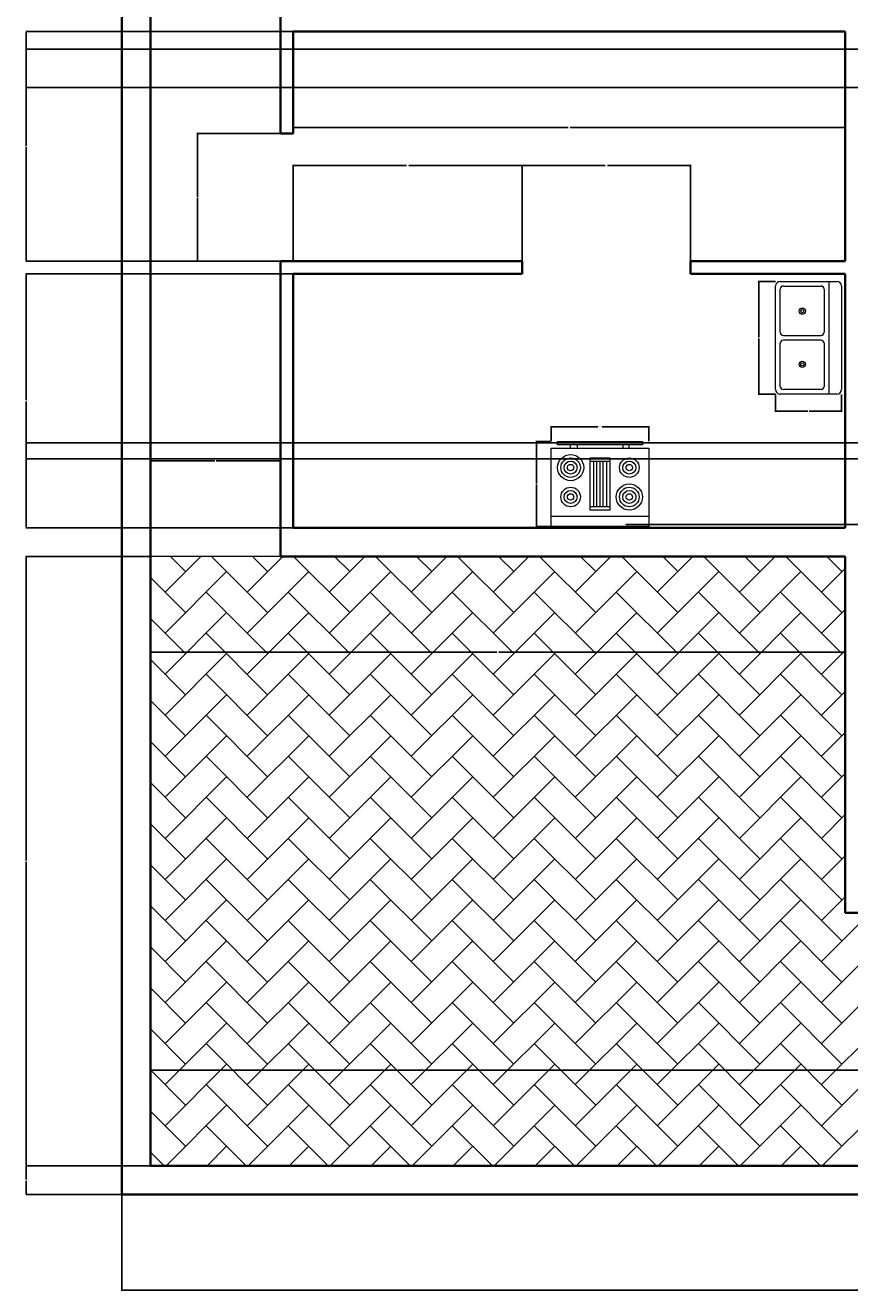
# Model space of a CAD drawing. Units: feet. Extents: x 2335 to 2876, y 491 to 1152.
# Tile 1 of 4: x 2335 to 2595, y 491 to 890. Entities that reach past the tile are written whole.
import ezdxf

# ---------------------------------------------------------------- set-up
doc = ezdxf.new("R2010")
doc.units = ezdxf.units.FT
for name, color, linetype, lineweight in [('A-ANNO-DIMS', 2, 'Continuous', 18), ('A-EQPM', 9, 'Continuous', 18), ('A-FLOR-FIXT', 9, 'Continuous', 18), ('A-WALL', 7, 'Continuous', 35), ('C-PROP', 3, 'Continuous', 35), ('C-PVMT', 8, 'Continuous', 18), ('C-PVMT-PATT', 252, 'Continuous', 13)]:
    doc.layers.add(name, color=color, linetype=linetype, lineweight=lineweight)
doc.styles.get("Standard").update_dxf_attribs({"font": 'arial.ttf'})
doc.dimstyles.get("Standard").update_dxf_attribs({"dimtxt": 0.18, "dimasz": 0.18, "dimexe": 0.18, "dimexo": 0.0625, "dimgap": 0.09, "dimtad": 0, "dimtih": 1, "dimtoh": 1, "dimdec": 4, "dimzin": 0, "dimdsep": 46, "dimlunit": 4, "dimtxsty": 'Standard', "dimcen": 0.09, "dimadec": 0, "dimazin": 0, "dimtfac": 1, "dimtdec": 4, "dimtofl": 0, "dimtmove": 0, "dimatfit": 3, "dimfxl": 1, "dimtolj": 1, "dimtzin": 0, "dimarcsym": 0})

# ---------------------------------------------------------------- blocks, each defined once
blk = doc.blocks.new('Range-Oven - 30 in top')
for p, q in [((0, -3), (30, -3)), ((12, -6), (18, -6)), ((13, -20), (13, -6)), ((14, -6), (14, -20)), ((15, -20), (15, -6)), ((16, -6), (16, -20)), ((17, -20), (17, -6)), ((18, -20), (12, -20)), ((6, -24), (6, -25)), ((8, -25), (8, -24)), ((22, -25), (22, -24)), ((24, -24), (24, -25))]:
    blk.add_line(p, q)
for points in [[(0, -24), (0, 0), (30, 0), (30, -24)], [(12, -21), (12, -5), (18, -5), (18, -21)], [(2, -26), (2, -25), (28, -25), (28, -26)]]:
    blk.add_lwpolyline(points, close=True)
for centre, radius in [((6, -9), 4), ((6, -9), 3), ((6, -9), 2), ((24, -9), 3), ((24, -9), 2), ((6, -9), 1), ((24, -9), 1), ((6, -18), 3), ((24, -18), 4), ((24, -18), 3), ((6, -18), 2), ((6, -18), 1), ((24, -18), 2), ((24, -18), 1)]:
    blk.add_circle(centre, radius)
blk = doc.blocks.new('Sink-double - 36 in top')
for p, q in [((-18, -4), (18, -4)), ((-0.75, -18.5), (-0.75, -6.5)), ((0.75, -6.5), (0.75, -18.5))]:
    blk.add_line(p, q)
for points in [[(-16.5, 0), (16.5, 0)], [(-18, -19.5), (-18, -1.5)], [(18, -1.5), (18, -19.5)], [(-16.5, -18.5), (-16.5, -6.5)], [(-15.5, -5.5), (-1.75, -5.5)], [(1.75, -5.5), (15.5, -5.5)], [(16.5, -6.5), (16.5, -18.5)], [(-1.75, -19.5), (-15.5, -19.5)], [(15.5, -19.5), (1.75, -19.5)], [(16.5, -21), (-16.5, -21)]]:
    blk.add_lwpolyline(points)
for centre, radius in [((-8.5, -12.5), 1), ((-8.5, -12.5), 0.5), ((8.5, -12.5), 1), ((8.5, -12.5), 0.5)]:
    blk.add_circle(centre, radius)
for centre, radius, start, end in [((-16.5, -1.5), 1.5, 90, 180), ((16.5, -1.5), 1.5, 0, 90), ((-15.5, -6.5), 1, 90, 180), ((-1.75, -6.5), 1, 0, 90), ((1.75, -6.5), 1, 90, 180), ((15.5, -6.5), 1, 0, 90), ((-16.5, -19.5), 1.5, 180, 270), ((-15.5, -18.5), 1, 180, 270), ((-1.75, -18.5), 1, 270, 0), ((1.75, -18.5), 1, 180, 270), ((15.5, -18.5), 1, 270, 0), ((16.5, -19.5), 1.5, 270, 0)]:
    blk.add_arc(centre, radius, start, end)
blk = doc.blocks.new('*D16')
at = {"layer": 'A-ANNO-DIMS', "color": 0, "lineweight": -2, "transparency": 16777216}
for p, q in [((2501.1, 758.74), (2501.1, 763.48)), ((2501.28, 763.3), (2515.84, 763.3)), ((2531.75, 763.3), (2517.2, 763.3)), ((2531.93, 758.74), (2531.93, 763.48))]:
    blk.add_line(p, q, dxfattribs=at)
at = {"layer": 'A-ANNO-DIMS', "color": 0, "transparency": 16777216}
for points in [[(2501.28, 763.33), (2501.28, 763.27), (2501.1, 763.3)], [(2531.75, 763.33), (2531.75, 763.27), (2531.93, 763.3)]]:
    blk.add_solid(points, dxfattribs=at)
at = {"layer": 'Defpoints', "color": 0, "transparency": 16777216}
for p in [(2501.1, 763.3), (2501.1, 758.68), (2531.93, 758.68)]:
    blk.add_point(p, dxfattribs=at)
at = {"layer": 'A-ANNO-DIMS', "color": 0, "transparency": 16777216, "insert": (2516.52, 763.3), "char_height": 0.18, "attachment_point": 5}
blk.add_mtext('\\A1;RANGE 31', dxfattribs=at)
blk = doc.blocks.new('*D17')
at = {"layer": 'A-ANNO-DIMS', "color": 0, "lineweight": -2, "transparency": 16777216}
for p, q in [((2501.04, 758.68), (2496.29, 758.68)), ((2496.47, 758.5), (2496.47, 745.5)), ((2496.47, 732.13), (2496.47, 745.14)), ((2501.04, 731.95), (2496.29, 731.95))]:
    blk.add_line(p, q, dxfattribs=at)
at = {"layer": 'A-ANNO-DIMS', "color": 0, "transparency": 16777216}
for points in [[(2496.44, 758.5), (2496.5, 758.5), (2496.47, 758.68)], [(2496.44, 732.13), (2496.5, 732.13), (2496.47, 731.95)]]:
    blk.add_solid(points, dxfattribs=at)
at = {"layer": 'Defpoints', "color": 0, "transparency": 16777216}
for p in [(2501.1, 758.68), (2496.47, 731.95), (2501.1, 731.95)]:
    blk.add_point(p, dxfattribs=at)
at = {"layer": 'A-ANNO-DIMS', "color": 0, "transparency": 16777216, "insert": (2496.47, 745.32), "char_height": 0.18, "attachment_point": 5}
blk.add_mtext('\\A1;27', dxfattribs=at)
blk = doc.blocks.new('*D18')
at = {"layer": 'A-ANNO-DIMS', "color": 0, "lineweight": -2, "transparency": 16777216}
for p, q in [((2571.83, 809.13), (2566.38, 809.13)), ((2566.56, 808.95), (2566.56, 791.54)), ((2566.56, 773.77), (2566.56, 791.18)), ((2571.83, 773.59), (2566.38, 773.59))]:
    blk.add_line(p, q, dxfattribs=at)
at = {"layer": 'A-ANNO-DIMS', "color": 0, "transparency": 16777216}
for points in [[(2566.53, 808.95), (2566.59, 808.95), (2566.56, 809.13)], [(2566.53, 773.77), (2566.59, 773.77), (2566.56, 773.59)]]:
    blk.add_solid(points, dxfattribs=at)
at = {"layer": 'Defpoints', "color": 0, "transparency": 16777216}
for p in [(2571.89, 809.13), (2566.56, 773.59), (2571.89, 773.59)]:
    blk.add_point(p, dxfattribs=at)
at = {"layer": 'A-ANNO-DIMS', "color": 0, "transparency": 16777216, "insert": (2566.56, 791.36), "char_height": 0.18, "attachment_point": 5}
blk.add_mtext('\\A1;SINK 36', dxfattribs=at)
blk = doc.blocks.new('*D19')
at = {"layer": 'A-ANNO-DIMS', "color": 0, "lineweight": -2, "transparency": 16777216}
for p, q in [((2571.89, 773.52), (2571.89, 768.07)), ((2592.63, 773.52), (2592.63, 768.07)), ((2572.07, 768.25), (2582.05, 768.25)), ((2592.45, 768.25), (2582.46, 768.25))]:
    blk.add_line(p, q, dxfattribs=at)
at = {"layer": 'A-ANNO-DIMS', "color": 0, "transparency": 16777216}
for points in [[(2572.07, 768.28), (2572.07, 768.22), (2571.89, 768.25)], [(2592.45, 768.28), (2592.45, 768.22), (2592.63, 768.25)]]:
    blk.add_solid(points, dxfattribs=at)
at = {"layer": 'Defpoints', "color": 0, "transparency": 16777216}
for p in [(2571.89, 773.59), (2592.63, 773.59), (2592.63, 768.25)]:
    blk.add_point(p, dxfattribs=at)
at = {"layer": 'A-ANNO-DIMS', "color": 0, "transparency": 16777216, "insert": (2582.26, 768.25), "char_height": 0.18, "attachment_point": 5}
blk.add_mtext('\\A1;21', dxfattribs=at)
blk = doc.blocks.new('*D24')
at = {"layer": 'A-ANNO-DIMS', "color": 0, "lineweight": -2, "transparency": 16777216}
for p, q in [((2365.8, 521.42), (2365.8, 491.16)), ((2845.8, 521.42), (2845.8, 491.16)), ((2365.98, 491.34), (2605.5, 491.34)), ((2845.62, 491.34), (2606.09, 491.34))]:
    blk.add_line(p, q, dxfattribs=at)
at = {"layer": 'A-ANNO-DIMS', "color": 0, "transparency": 16777216}
for points in [[(2365.98, 491.37), (2365.98, 491.31), (2365.8, 491.34)], [(2845.62, 491.37), (2845.62, 491.31), (2845.8, 491.34)]]:
    blk.add_solid(points, dxfattribs=at)
at = {"layer": 'Defpoints', "color": 0, "transparency": 16777216}
for p in [(2365.8, 521.49), (2845.8, 521.49), (2845.8, 491.34)]:
    blk.add_point(p, dxfattribs=at)
at = {"layer": 'A-ANNO-DIMS', "color": 0, "transparency": 16777216, "insert": (2605.8, 491.34), "char_height": 0.18, "attachment_point": 5}
blk.add_mtext('\\A1;480', dxfattribs=at)
blk = doc.blocks.new('*D26')
at = {"layer": 'A-ANNO-DIMS', "color": 0, "lineweight": -2, "transparency": 16777216}
for p, q in [((2374.8, 530.55), (2374.8, 560.82)), ((2374.98, 560.64), (2605.51, 560.64)), ((2836.62, 560.64), (2606.09, 560.64)), ((2836.8, 530.55), (2836.8, 560.82))]:
    blk.add_line(p, q, dxfattribs=at)
at = {"layer": 'A-ANNO-DIMS', "color": 0, "transparency": 16777216}
for points in [[(2374.98, 560.67), (2374.98, 560.61), (2374.8, 560.64)], [(2836.62, 560.67), (2836.62, 560.61), (2836.8, 560.64)]]:
    blk.add_solid(points, dxfattribs=at)
at = {"layer": 'Defpoints', "color": 0, "transparency": 16777216}
for p in [(2836.8, 560.64), (2374.8, 530.49), (2836.8, 530.49)]:
    blk.add_point(p, dxfattribs=at)
at = {"layer": 'A-ANNO-DIMS', "color": 0, "transparency": 16777216, "insert": (2605.8, 560.64), "char_height": 0.18, "attachment_point": 5}
blk.add_mtext('\\A1;462', dxfattribs=at)
blk = doc.blocks.new('*D27')
at = {"layer": 'A-ANNO-DIMS', "color": 0, "lineweight": -2, "transparency": 16777216}
for p, q in [((2374.8, 722.42), (2374.8, 692.16)), ((2593.8, 722.42), (2593.8, 692.16)), ((2374.98, 692.34), (2484.01, 692.34)), ((2593.62, 692.34), (2484.59, 692.34))]:
    blk.add_line(p, q, dxfattribs=at)
at = {"layer": 'A-ANNO-DIMS', "color": 0, "transparency": 16777216}
for points in [[(2374.98, 692.37), (2374.98, 692.31), (2374.8, 692.34)], [(2593.62, 692.37), (2593.62, 692.31), (2593.8, 692.34)]]:
    blk.add_solid(points, dxfattribs=at)
at = {"layer": 'Defpoints', "color": 0, "transparency": 16777216}
for p in [(2374.8, 722.49), (2593.8, 722.49), (2374.8, 692.34)]:
    blk.add_point(p, dxfattribs=at)
at = {"layer": 'A-ANNO-DIMS', "color": 0, "transparency": 16777216, "insert": (2484.3, 692.34), "char_height": 0.18, "attachment_point": 5}
blk.add_mtext('\\A1;219', dxfattribs=at)
blk = doc.blocks.new('*D28')
at = {"layer": 'A-ANNO-DIMS', "color": 0, "lineweight": -2, "transparency": 16777216}
for p, q in [((2374.73, 722.49), (2335.47, 722.49)), ((2335.65, 722.31), (2335.65, 626.67)), ((2335.65, 530.67), (2335.65, 626.31)), ((2374.73, 530.49), (2335.47, 530.49))]:
    blk.add_line(p, q, dxfattribs=at)
at = {"layer": 'A-ANNO-DIMS', "color": 0, "transparency": 16777216}
for points in [[(2335.62, 722.31), (2335.68, 722.31), (2335.65, 722.49)], [(2335.62, 530.67), (2335.68, 530.67), (2335.65, 530.49)]]:
    blk.add_solid(points, dxfattribs=at)
at = {"layer": 'Defpoints', "color": 0, "transparency": 16777216}
for p in [(2335.65, 722.49), (2374.8, 722.49), (2374.8, 530.49)]:
    blk.add_point(p, dxfattribs=at)
at = {"layer": 'A-ANNO-DIMS', "color": 0, "transparency": 16777216, "insert": (2335.65, 626.49), "char_height": 0.18, "attachment_point": 5}
blk.add_mtext('\\A1;192', dxfattribs=at)
blk = doc.blocks.new('*D29')
at = {"layer": 'A-ANNO-DIMS', "color": 0, "lineweight": -2, "transparency": 16777216}
for p, q in [((2374.73, 530.49), (2335.47, 530.49)), ((2335.65, 530.31), (2335.65, 526.17)), ((2335.65, 521.67), (2335.65, 525.81)), ((2365.73, 521.49), (2335.47, 521.49))]:
    blk.add_line(p, q, dxfattribs=at)
at = {"layer": 'A-ANNO-DIMS', "color": 0, "transparency": 16777216}
for points in [[(2335.62, 530.31), (2335.68, 530.31), (2335.65, 530.49)], [(2335.62, 521.67), (2335.68, 521.67), (2335.65, 521.49)]]:
    blk.add_solid(points, dxfattribs=at)
at = {"layer": 'Defpoints', "color": 0, "transparency": 16777216}
for p in [(2335.65, 530.49), (2374.8, 530.49), (2365.8, 521.49)]:
    blk.add_point(p, dxfattribs=at)
at = {"layer": 'A-ANNO-DIMS', "color": 0, "transparency": 16777216, "insert": (2335.65, 525.99), "char_height": 0.18, "attachment_point": 5}
blk.add_mtext('\\A1;9', dxfattribs=at)
blk = doc.blocks.new('*D39')
at = {"layer": 'A-ANNO-DIMS', "color": 0, "lineweight": -2, "transparency": 16777216}
for p, q in [((2760.82, 882.23), (2335.47, 882.23)), ((2335.65, 882.05), (2335.65, 876.41)), ((2335.65, 870.41), (2335.65, 876.05)), ((2760.82, 870.23), (2335.47, 870.23))]:
    blk.add_line(p, q, dxfattribs=at)
at = {"layer": 'A-ANNO-DIMS', "color": 0, "transparency": 16777216}
for points in [[(2335.62, 882.05), (2335.68, 882.05), (2335.65, 882.23)], [(2335.62, 870.41), (2335.68, 870.41), (2335.65, 870.23)]]:
    blk.add_solid(points, dxfattribs=at)
at = {"layer": 'Defpoints', "color": 0, "transparency": 16777216}
for p in [(2335.65, 882.23), (2760.88, 882.23), (2760.88, 870.23)]:
    blk.add_point(p, dxfattribs=at)
at = {"layer": 'A-ANNO-DIMS', "color": 0, "transparency": 16777216, "insert": (2335.65, 876.23), "char_height": 0.18, "attachment_point": 5}
blk.add_mtext('\\A1;12', dxfattribs=at)
blk = doc.blocks.new('*D43')
at = {"layer": 'A-ANNO-DIMS', "color": 0, "lineweight": -2, "transparency": 16777216}
for p, q in [((2760.82, 758.23), (2335.47, 758.23)), ((2335.65, 758.05), (2335.65, 755.91)), ((2335.65, 753.41), (2335.65, 755.54)), ((2760.82, 753.23), (2335.47, 753.23))]:
    blk.add_line(p, q, dxfattribs=at)
at = {"layer": 'A-ANNO-DIMS', "color": 0, "transparency": 16777216}
for points in [[(2335.62, 758.05), (2335.68, 758.05), (2335.65, 758.23)], [(2335.62, 753.41), (2335.68, 753.41), (2335.65, 753.23)]]:
    blk.add_solid(points, dxfattribs=at)
at = {"layer": 'Defpoints', "color": 0, "transparency": 16777216}
for p in [(2335.65, 758.23), (2760.88, 758.23), (2760.88, 753.23)]:
    blk.add_point(p, dxfattribs=at)
at = {"layer": 'A-ANNO-DIMS', "color": 0, "transparency": 16777216, "insert": (2335.65, 755.73), "char_height": 0.18, "attachment_point": 5}
blk.add_mtext('\\A1;5', dxfattribs=at)
blk = doc.blocks.new('*D44')
at = {"layer": 'A-ANNO-DIMS', "color": 0, "lineweight": -2, "transparency": 16777216}
for p, q in [((2374.8, 722.55), (2374.8, 752.82)), ((2374.98, 752.64), (2395.09, 752.64)), ((2415.62, 752.64), (2395.5, 752.64)), ((2415.8, 722.55), (2415.8, 752.82))]:
    blk.add_line(p, q, dxfattribs=at)
at = {"layer": 'A-ANNO-DIMS', "color": 0, "transparency": 16777216}
for points in [[(2374.98, 752.67), (2374.98, 752.61), (2374.8, 752.64)], [(2415.62, 752.67), (2415.62, 752.61), (2415.8, 752.64)]]:
    blk.add_solid(points, dxfattribs=at)
at = {"layer": 'Defpoints', "color": 0, "transparency": 16777216}
for p in [(2415.8, 752.64), (2374.8, 722.49), (2415.8, 722.49)]:
    blk.add_point(p, dxfattribs=at)
at = {"layer": 'A-ANNO-DIMS', "color": 0, "transparency": 16777216, "insert": (2395.3, 752.64), "char_height": 0.18, "attachment_point": 5}
blk.add_mtext('\\A1;41', dxfattribs=at)
blk = doc.blocks.new('*D45')
at = {"layer": 'A-ANNO-DIMS', "color": 0, "lineweight": -2, "transparency": 16777216}
for p, q in [((2419.73, 811.49), (2335.47, 811.49)), ((2335.65, 811.31), (2335.65, 771.67)), ((2335.65, 731.67), (2335.65, 771.31)), ((2419.73, 731.49), (2335.47, 731.49))]:
    blk.add_line(p, q, dxfattribs=at)
at = {"layer": 'A-ANNO-DIMS', "color": 0, "transparency": 16777216}
for points in [[(2335.62, 811.31), (2335.68, 811.31), (2335.65, 811.49)], [(2335.62, 731.67), (2335.68, 731.67), (2335.65, 731.49)]]:
    blk.add_solid(points, dxfattribs=at)
at = {"layer": 'Defpoints', "color": 0, "transparency": 16777216}
for p in [(2335.65, 811.49), (2419.8, 811.49), (2419.8, 731.49)]:
    blk.add_point(p, dxfattribs=at)
at = {"layer": 'A-ANNO-DIMS', "color": 0, "transparency": 16777216, "insert": (2335.65, 771.49), "char_height": 0.18, "attachment_point": 5}
blk.add_mtext('\\A1;80', dxfattribs=at)
blk = doc.blocks.new('*D46')
at = {"layer": 'A-ANNO-DIMS', "color": 0, "lineweight": -2, "transparency": 16777216}
for p, q in [((2419.8, 815.55), (2419.8, 845.82)), ((2419.98, 845.64), (2455.53, 845.64)), ((2491.83, 845.64), (2456.28, 845.64)), ((2492.01, 815.55), (2492.01, 845.82))]:
    blk.add_line(p, q, dxfattribs=at)
at = {"layer": 'A-ANNO-DIMS', "color": 0, "transparency": 16777216}
for points in [[(2419.98, 845.67), (2419.98, 845.61), (2419.8, 845.64)], [(2491.83, 845.67), (2491.83, 845.61), (2492.01, 845.64)]]:
    blk.add_solid(points, dxfattribs=at)
at = {"layer": 'Defpoints', "color": 0, "transparency": 16777216}
for p in [(2492.01, 845.64), (2419.8, 815.49), (2492.01, 815.49)]:
    blk.add_point(p, dxfattribs=at)
at = {"layer": 'A-ANNO-DIMS', "color": 0, "transparency": 16777216, "insert": (2455.9, 845.64), "char_height": 0.18, "attachment_point": 5}
blk.add_mtext('\\A1;72.21', dxfattribs=at)
blk = doc.blocks.new('*D47')
at = {"layer": 'A-ANNO-DIMS', "color": 0, "lineweight": -2, "transparency": 16777216}
for p, q in [((2492.01, 815.55), (2492.01, 845.82)), ((2492.19, 845.64), (2518.14, 845.64)), ((2544.88, 845.64), (2518.92, 845.64)), ((2545.06, 815.55), (2545.06, 845.82))]:
    blk.add_line(p, q, dxfattribs=at)
at = {"layer": 'A-ANNO-DIMS', "color": 0, "transparency": 16777216}
for points in [[(2492.19, 845.67), (2492.19, 845.61), (2492.01, 845.64)], [(2544.88, 845.67), (2544.88, 845.61), (2545.06, 845.64)]]:
    blk.add_solid(points, dxfattribs=at)
at = {"layer": 'Defpoints', "color": 0, "transparency": 16777216}
for p in [(2545.06, 845.64), (2492.01, 815.49), (2545.06, 815.49)]:
    blk.add_point(p, dxfattribs=at)
at = {"layer": 'A-ANNO-DIMS', "color": 0, "transparency": 16777216, "insert": (2518.53, 845.64), "char_height": 0.18, "attachment_point": 5}
blk.add_mtext('\\A1;53.05', dxfattribs=at)
blk = doc.blocks.new('*D48')
at = {"layer": 'A-ANNO-DIMS', "color": 0, "lineweight": -2, "transparency": 16777216}
for p, q in [((2419.73, 887.8), (2335.47, 887.8)), ((2335.65, 887.62), (2335.65, 851.82)), ((2335.65, 815.67), (2335.65, 851.46)), ((2419.73, 815.49), (2335.47, 815.49))]:
    blk.add_line(p, q, dxfattribs=at)
at = {"layer": 'A-ANNO-DIMS', "color": 0, "transparency": 16777216}
for points in [[(2335.62, 887.62), (2335.68, 887.62), (2335.65, 887.8)], [(2335.62, 815.67), (2335.68, 815.67), (2335.65, 815.49)]]:
    blk.add_solid(points, dxfattribs=at)
at = {"layer": 'Defpoints', "color": 0, "transparency": 16777216}
for p in [(2335.65, 887.8), (2419.8, 887.8), (2419.8, 815.49)]:
    blk.add_point(p, dxfattribs=at)
at = {"layer": 'A-ANNO-DIMS', "color": 0, "transparency": 16777216, "insert": (2335.65, 851.64), "char_height": 0.18, "attachment_point": 5}
blk.add_mtext('\\A1;72.31', dxfattribs=at)
blk = doc.blocks.new('*D49')
at = {"layer": 'A-ANNO-DIMS', "color": 0, "lineweight": -2, "transparency": 16777216}
for p, q in [((2419.73, 855.76), (2389.47, 855.76)), ((2389.65, 855.58), (2389.65, 835.8)), ((2389.65, 815.67), (2389.65, 835.44)), ((2419.73, 815.49), (2389.47, 815.49))]:
    blk.add_line(p, q, dxfattribs=at)
at = {"layer": 'A-ANNO-DIMS', "color": 0, "transparency": 16777216}
for points in [[(2389.68, 855.58), (2389.62, 855.58), (2389.65, 855.76)], [(2389.68, 815.67), (2389.62, 815.67), (2389.65, 815.49)]]:
    blk.add_solid(points, dxfattribs=at)
at = {"layer": 'Defpoints', "color": 0, "transparency": 16777216}
for p in [(2389.65, 855.76), (2419.8, 855.76), (2419.8, 815.49)]:
    blk.add_point(p, dxfattribs=at)
at = {"layer": 'A-ANNO-DIMS', "color": 0, "transparency": 16777216, "insert": (2389.65, 835.62), "char_height": 0.18, "attachment_point": 5}
blk.add_mtext('\\A1;40.27', dxfattribs=at)
blk = doc.blocks.new('*D54')
at = {"layer": 'A-ANNO-DIMS', "color": 0, "lineweight": -2, "transparency": 16777216}
for p, q in [((2419.8, 887.74), (2419.8, 857.47)), ((2593.8, 887.74), (2593.8, 857.47)), ((2419.98, 857.65), (2506.52, 857.65)), ((2593.62, 857.65), (2507.08, 857.65))]:
    blk.add_line(p, q, dxfattribs=at)
at = {"layer": 'A-ANNO-DIMS', "color": 0, "transparency": 16777216}
for points in [[(2419.98, 857.68), (2419.98, 857.62), (2419.8, 857.65)], [(2593.62, 857.68), (2593.62, 857.62), (2593.8, 857.65)]]:
    blk.add_solid(points, dxfattribs=at)
at = {"layer": 'Defpoints', "color": 0, "transparency": 16777216}
for p in [(2419.8, 887.8), (2593.8, 887.8), (2419.8, 857.65)]:
    blk.add_point(p, dxfattribs=at)
at = {"layer": 'A-ANNO-DIMS', "color": 0, "transparency": 16777216, "insert": (2506.8, 857.65), "char_height": 0.18, "attachment_point": 5}
blk.add_mtext('\\A1;174', dxfattribs=at)
blk = doc.blocks.new('*D70')
at = {"layer": 'A-ANNO-DIMS', "color": 0, "lineweight": -2, "transparency": 16777216}
for p, q in [((2526.66, 732.49), (2605.99, 732.49)), ((2738.6, 732.49), (2738.78, 732.49)), ((2738.69, 732.4), (2738.69, 732.58))]:
    blk.add_line(p, q, dxfattribs=at)
at = {"layer": 'A-ANNO-DIMS', "color": 0, "transparency": 16777216}
blk.add_solid([(2605.99, 732.52), (2605.99, 732.46), (2606.17, 732.49)], dxfattribs=at)
at = {"layer": 'Defpoints', "color": 0, "transparency": 16777216}
for p in [(2606.17, 732.49), (2738.69, 732.49)]:
    blk.add_point(p, dxfattribs=at)
at = {"layer": 'A-ANNO-DIMS', "color": 0, "transparency": 16777216, "insert": (2526.11, 732.49), "char_height": 0.18, "attachment_point": 5}
blk.add_mtext('\\A1;R132.52', dxfattribs=at)
blk = doc.blocks.new('*D71')
at = {"layer": 'A-ANNO-DIMS', "color": 0, "lineweight": -2, "transparency": 16777216}
for p, q in [((2524.65, 732.49), (2599.43, 732.49)), ((2724.44, 732.49), (2724.62, 732.49)), ((2724.53, 732.4), (2724.53, 732.58))]:
    blk.add_line(p, q, dxfattribs=at)
at = {"layer": 'A-ANNO-DIMS', "color": 0, "transparency": 16777216}
blk.add_solid([(2599.43, 732.52), (2599.43, 732.46), (2599.61, 732.49)], dxfattribs=at)
at = {"layer": 'Defpoints', "color": 0, "transparency": 16777216}
for p in [(2599.61, 732.49), (2724.53, 732.49)]:
    blk.add_point(p, dxfattribs=at)
at = {"layer": 'A-ANNO-DIMS', "color": 0, "transparency": 16777216, "insert": (2524.1, 732.49), "char_height": 0.18, "attachment_point": 5}
blk.add_mtext('\\A1;R124.93', dxfattribs=at)

msp = doc.modelspace()

# ---------------------------------------------------------------- hatches: boundary and pattern name
at = {"layer": 'C-PVMT-PATT'}
h = msp.add_hatch(dxfattribs=at)
h.set_pattern_fill('AR-HBONE', color=256, scale=0.09)
h.paths.add_polyline_path([(2593.7974, 722.4872), (2419.7974, 722.4872), (2415.7974, 722.4872), (2374.7967, 722.4872), (2374.7967, 530.4872), (2593.7974, 530.4872), (2597.7974, 530.4872), (2836.7967, 530.4872), (2836.7967, 610.2261), (2729.1837, 610.2261), (2652.5752, 610.2261), (2597.7974, 610.2261), (2593.7974, 610.2261)])

# ---------------------------------------------------------------- linework, layer by layer
at = {"layer": 'A-WALL'}
for p, q in [((2415.7974, 855.7568), (2415.7974, 1081.7975)), ((2419.7969, 855.7568), (2419.7969, 887.7975)), ((2419.7974, 887.7975), (2593.7974, 887.7975)), ((2593.7974, 887.7975), (2593.7974, 815.4872)), ((2415.7974, 855.7568), (2419.7969, 855.7568)), ((2415.7974, 722.4872), (2415.7974, 815.4872)), ((2419.7967, 815.4872), (2415.7974, 815.4872)), ((2419.7974, 815.4872), (2492.0051, 815.4872)), ((2464.7974, 815.4872), (2492.0051, 815.4872)), ((2492.0051, 811.4872), (2492.0051, 815.4872)), ((2545.0559, 815.4872), (2545.0559, 811.4872)), ((2545.0559, 815.4872), (2593.7974, 815.4872)), ((2545.0559, 815.4872), (2593.7974, 815.4872)), ((2419.7974, 811.4872), (2492.0051, 811.4872)), ((2419.7974, 811.4872), (2419.7974, 731.4872)), ((2545.0559, 811.4872), (2593.7974, 811.4872)), ((2593.7974, 811.4872), (2593.7974, 731.4872)), ((2593.7974, 811.4872), (2593.7974, 784.7975)), ((2419.7974, 731.4872), (2593.7974, 731.4872)), ((2419.7974, 722.4872), (2415.7974, 722.4872)), ((2593.7974, 722.4872), (2419.7974, 722.4872)), ((2593.7974, 722.4872), (2593.7974, 610.2261)), ((2597.7974, 610.2261), (2593.7974, 610.2261))]:
    msp.add_line(p, q, dxfattribs=at)
at = {"layer": 'C-PROP'}
msp.add_line((2593.7974, 530.4872), (2597.7974, 530.4872), dxfattribs=at)
msp.add_lwpolyline([(2845.7967, 521.4872), (2845.7967, 1121.4872), (2365.7967, 1121.4872), (2365.7967, 521.4872)], close=True, dxfattribs=at)
msp.add_lwpolyline([(2697.7974, 1112.4872), (2374.7967, 1112.4872), (2374.7967, 530.4872), (2593.7974, 530.4872)], dxfattribs=at)
at = {"layer": 'C-PVMT'}
msp.add_line((2415.7974, 722.4872), (2374.7967, 722.4872), dxfattribs=at)

# ---------------------------------------------------------------- block references
at = {"layer": 'A-EQPM', "xscale": 1.027898850187762, "yscale": 1.027898850187762, "zscale": 1.027898850187762, "rotation": 180}
msp.add_blockref('Range-Oven - 30 in top', (2531.935, 731.9529), dxfattribs=at)
at = {"layer": 'A-FLOR-FIXT', "xscale": 0.9874339846236208, "yscale": 0.9874339846236208, "zscale": 0.9874339846236208, "rotation": 270}
msp.add_blockref('Sink-double - 36 in top', (2592.6259, 791.3588), dxfattribs=at)

# ---------------------------------------------------------------- dimensions: what is measured, and where the dimension line sits
at = {"layer": 'A-ANNO-DIMS'}
for base, p1, p2, angle, override, picture, middle in [((2335.6467, 887.7975), (2419.7974, 815.4872), (2419.7974, 887.7975), 90, {"dimdec": 2, "dimlfac": 1, "dimrnd": 0, "dimzin": 0, "dimdsep": 46, "dimlunit": 2}, '*D48', (2335.6467, 851.6423)), ((2419.7974, 857.6475), (2593.7974, 887.7975), (2419.7974, 887.7975), 180, {"dimdec": 0, "dimlfac": 1, "dimrnd": 0, "dimzin": 0, "dimdsep": 46, "dimlunit": 2}, '*D54', (2506.7974, 857.6475)), ((2335.6467, 882.2261), (2760.8783, 870.2261), (2760.8783, 882.2261), 90, {"dimdec": 0, "dimlfac": 1, "dimrnd": 0, "dimzin": 0, "dimdsep": 46, "dimlunit": 2}, '*D39', (2335.6467, 876.2261)), ((2389.6469, 855.7564), (2419.7974, 815.4872), (2419.7969, 855.7568), 90.00067, {"dimdec": 2, "dimlfac": 1, "dimrnd": 0, "dimzin": 0, "dimdsep": 46, "dimlunit": 2}, '*D49', (2389.6472, 835.6216)), ((2335.6467, 811.4872), (2419.7974, 731.4872), (2419.7974, 811.4872), 90, {"dimdec": 0, "dimlfac": 1, "dimrnd": 0, "dimzin": 0, "dimdsep": 46, "dimlunit": 2}, '*D45', (2335.6467, 771.4872)), ((2335.6467, 758.2261), (2760.8783, 753.2261), (2760.8783, 758.2261), 90, {"dimdec": 0, "dimlfac": 1, "dimrnd": 0, "dimzin": 0, "dimdsep": 46, "dimlunit": 2}, '*D43', (2335.6467, 755.7261)), ((2496.4725, 731.9529), (2501.098, 758.6783), (2501.098, 731.9529), 270, {"dimdec": 0, "dimlfac": 1, "dimrnd": 0, "dimzin": 0, "dimdsep": 46, "dimlunit": 2}, '*D17', (2496.4725, 745.3156)), ((2335.6467, 722.4872), (2374.7967, 530.4872), (2374.7967, 722.4872), 90, {"dimdec": 0, "dimlfac": 1, "dimrnd": 0, "dimzin": 0, "dimdsep": 46, "dimlunit": 2}, '*D28', (2335.6467, 626.4872)), ((2374.7967, 692.3372), (2593.7974, 722.4872), (2374.7967, 722.4872), 180, {"dimdec": 0, "dimlfac": 1, "dimrnd": 0, "dimzin": 0, "dimdsep": 46, "dimlunit": 2}, '*D27', (2484.297, 692.3372)), ((2836.7967, 560.6372), (2374.7967, 530.4872), (2836.7967, 530.4872), 0, {"dimdec": 0, "dimlfac": 1, "dimrnd": 0, "dimzin": 0, "dimdsep": 46, "dimlunit": 2}, '*D26', (2605.7967, 560.6372)), ((2335.6467, 530.4872), (2365.7967, 521.4872), (2374.7967, 530.4872), 90, {"dimdec": 0, "dimlfac": 1, "dimrnd": 0, "dimzin": 0, "dimdsep": 46, "dimlunit": 2}, '*D29', (2335.6467, 525.9872))]:
    dim = msp.add_linear_dim(base=base, p1=p1, p2=p2, angle=angle, dimstyle='Standard', override=override, dxfattribs=at)
    dim.commit()
    dim.dimension.update_dxf_attribs({"geometry": picture, "text_midpoint": middle})
for base, p1, p2, override, picture, middle in [((2492.0051, 845.6372), (2419.7974, 815.4872), (2492.0051, 815.4872), {"dimdec": 2, "dimlfac": 1, "dimrnd": 0, "dimzin": 0, "dimdsep": 46, "dimlunit": 2}, '*D46', (2455.9013, 845.6372)), ((2545.0559, 845.6372), (2492.0051, 815.4872), (2545.0559, 815.4872), {"dimdec": 2, "dimlfac": 1, "dimrnd": 0, "dimzin": 0, "dimdsep": 46, "dimlunit": 2}, '*D47', (2518.5305, 845.6372)), ((2592.6259, 768.2529), (2571.8897, 773.585), (2592.6259, 773.585), {"dimdec": 0, "dimlfac": 1, "dimrnd": 0, "dimzin": 0, "dimdsep": 46, "dimlunit": 2}, '*D19', (2582.2578, 768.2529)), ((2415.7974, 752.6372), (2374.7967, 722.4872), (2415.7974, 722.4872), {"dimdec": 0, "dimlfac": 1, "dimrnd": 0, "dimzin": 0, "dimdsep": 46, "dimlunit": 2}, '*D44', (2395.297, 752.6372)), ((2845.7967, 491.3372), (2365.7967, 521.4872), (2845.7967, 521.4872), {"dimdec": 0, "dimlfac": 1, "dimrnd": 0, "dimzin": 0, "dimdsep": 46, "dimlunit": 2}, '*D24', (2605.7967, 491.3372))]:
    dim = msp.add_linear_dim(base=base, p1=p1, p2=p2, dimstyle='Standard', override=override, dxfattribs=at)
    dim.commit()
    dim.dimension.update_dxf_attribs({"geometry": picture, "text_midpoint": middle})
for base, p1, p2, angle, text, picture, middle in [((2566.5576, 773.585), (2571.8897, 809.1326), (2571.8897, 773.585), 270, 'SINK <>', '*D18', (2566.5576, 791.3588)), ((2501.098, 763.3038), (2531.935, 758.6783), (2501.098, 758.6783), 180, 'RANGE <>', '*D16', (2516.5165, 763.3038))]:
    dim = msp.add_linear_dim(base=base, p1=p1, p2=p2, angle=angle, text=text, dimstyle='Standard', override={"dimdec": 0, "dimlfac": 1, "dimrnd": 0, "dimzin": 0, "dimdsep": 46, "dimlunit": 2}, dxfattribs=at)
    dim.commit()
    dim.dimension.update_dxf_attribs({"geometry": picture, "text_midpoint": middle})
for center, mpoint, picture, middle in [((2724.5349, 732.4927), (2599.6087, 732.493), '*D71', (2524.6529, 732.4932)), ((2738.6915, 732.4927), (2606.1693, 732.493), '*D70', (2526.656, 732.4932))]:
    dim = msp.add_radius_dim(center=center, mpoint=mpoint, dimstyle='Standard', override={"dimdec": 2, "dimlfac": 1, "dimrnd": 0, "dimzin": 0, "dimdsep": 46, "dimlunit": 2}, dxfattribs=at)
    dim.commit()
    dim.dimension.update_dxf_attribs({"geometry": picture, "text_midpoint": middle, "dimtype": 164})

doc.saveas('drawing.dxf')
